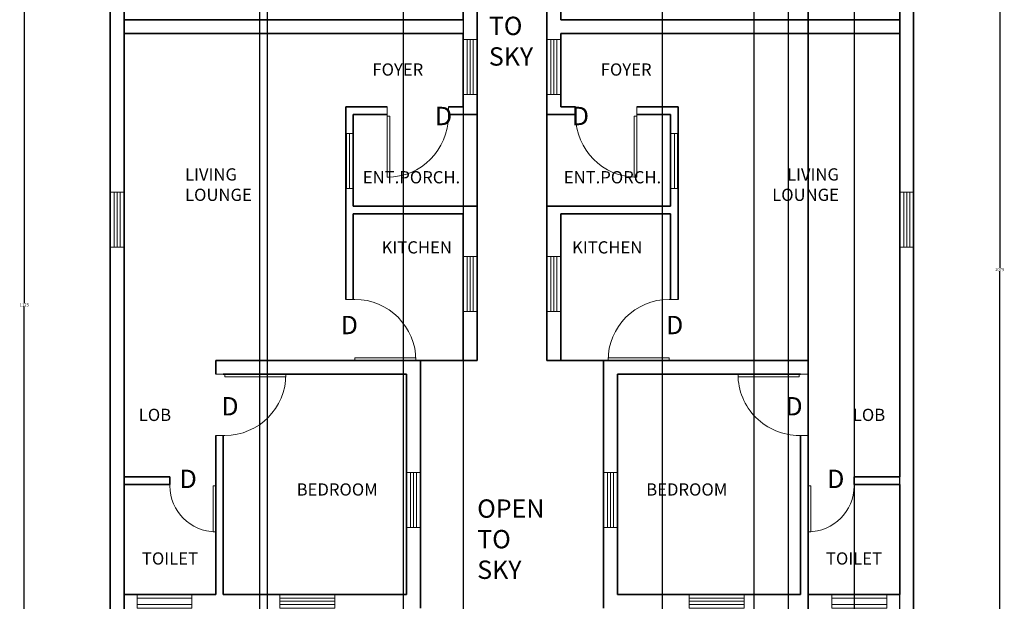
# Model space of a CAD drawing. Units: inches. Extents: x 190 to 836, y -241 to 999.
# Tile 5 of 9: x 191 to 836, y 185 to 566. Entities that reach past the tile are written whole.
import ezdxf

# ---------------------------------------------------------------- set-up
doc = ezdxf.new("R2010")
doc.units = ezdxf.units.IN
doc.header["$MEASUREMENT"] = 0
for name, color, linetype, lineweight in [('A-ANNO-DIMS', 2, 'Continuous', 18), ('A-ANNO-TEXT', 7, 'Continuous', 18), ('A-AREA-IDEN', 7, 'Continuous', 18), ('A-DOOR', 3, 'Continuous', 18), ('A-GLAZ', 4, 'Continuous', 18), ('A-WALL', 7, 'Continuous', 35)]:
    doc.layers.add(name, color=color, linetype=linetype, lineweight=lineweight)
doc.styles.get("Standard").update_dxf_attribs({"font": 'arial.ttf'})
doc.dimstyles.get("Standard").update_dxf_attribs({"dimtxt": 2, "dimasz": 2, "dimexe": 0.18, "dimexo": 0.0625, "dimgap": 0.09, "dimtad": 0, "dimtih": 1, "dimtoh": 1, "dimdec": 0, "dimzin": 0, "dimdsep": 46, "dimlunit": 3, "dimtxsty": 'Standard', "dimcen": 0.09, "dimadec": 0, "dimazin": 0, "dimtfac": 1, "dimtdec": 0, "dimtofl": 0, "dimtmove": 0, "dimatfit": 3, "dimfxl": 1, "dimtolj": 1, "dimtzin": 0, "dimarcsym": 0})

# ---------------------------------------------------------------- blocks, each defined once
blk = doc.blocks.new('*U2')
for p, q in [((0, 0), (0, 6)), ((40, 0), (40, 6))]:
    blk.add_line(p, q)
blk.add_lwpolyline([(0, 0), (0, -40), (1.75, -40), (1.75, 0)], close=True)
blk.add_arc((0, 0), 40, 270, 360)
blk = doc.blocks.new('*U4')
for p, q in [((-40, 0), (-40, 6)), ((0, 0), (0, 6))]:
    blk.add_line(p, q)
blk.add_lwpolyline([(0, 0), (0, -40), (-1.75, -40), (-1.75, 0)], close=True)
blk.add_arc((0, 0), 40, 180, 270)
blk = doc.blocks.new('*U5')
for p, q in [((0, 0), (0, -6)), ((40, 0), (40, -6))]:
    blk.add_line(p, q)
blk.add_lwpolyline([(0, 0), (0, 40), (1.75, 40), (1.75, 0)], close=True)
blk.add_arc((0, 0), 40, 0, 90)
blk = doc.blocks.new('*U3')
for p, q in [((-30, 0), (-30, -6)), ((0, 0), (0, -6))]:
    blk.add_line(p, q)
blk.add_lwpolyline([(0, 0), (0, 30), (-1.75, 30), (-1.75, 0)], close=True)
blk.add_arc((0, 0), 30, 90, 180)
blk = doc.blocks.new('WIN-36IN-9IN-3LINE')
for p, q in [((2.5, 36), (2.5, 0)), ((4.5, 36), (4.5, 0)), ((6.5, 36), (6.5, 0))]:
    blk.add_line(p, q)
blk.add_lwpolyline([(0, 0), (9, 0), (9, 36), (0, 36)], close=True)
blk = doc.blocks.new('WIN-36IN-9IN-2LINE')
for p, q in [((0, 6.5), (36, 6.5)), ((0, 2.5), (36, 2.5))]:
    blk.add_line(p, q)
blk.add_lwpolyline([(36, 0), (36, 9), (0, 9), (0, 0)], close=True)
blk = doc.blocks.new('WIN-36IN-5IN-PARTITION')
for p, q in [((5, 36), (0, 36)), ((0.5, 36), (0.5, 0)), ((2.5, 36), (2.5, 0)), ((5, 0), (5, 36)), ((0, 0), (5, 0))]:
    blk.add_line(p, q)
blk = doc.blocks.new('*D17')
at = {"layer": 'A-ANNO-DIMS', "color": 0, "lineweight": -2, "transparency": 16777216}
for p, q in [((250.38, 941.53), (193.96, 941.53)), ((194.14, 939.53), (194.14, 380.14)), ((194.14, -181.47), (194.14, 377.92)), ((447.38, -183.47), (193.96, -183.47))]:
    blk.add_line(p, q, dxfattribs=at)
at = {"layer": 'A-ANNO-DIMS', "color": 0, "transparency": 16777216}
for points in [[(193.8, 939.53), (194.47, 939.53), (194.14, 941.53)], [(193.8, -181.47), (194.47, -181.47), (194.14, -183.47)]]:
    blk.add_solid(points, dxfattribs=at)
at = {"layer": 'Defpoints', "color": 0, "transparency": 16777216}
for p in [(194.14, 941.53), (250.44, 941.53), (447.44, -183.47)]:
    blk.add_point(p, dxfattribs=at)
at = {"layer": 'A-ANNO-DIMS', "color": 0, "transparency": 16777216, "insert": (194.14, 379.03), "char_height": 2, "attachment_point": 5}
blk.add_mtext('\\A1;1125', dxfattribs=at)
blk = doc.blocks.new('*D18')
at = {"layer": 'A-ANNO-DIMS', "color": 0, "lineweight": -2, "transparency": 16777216}
for p, q in [((776.5, 941.53), (832.94, 941.53)), ((832.76, 939.53), (832.76, 403.14)), ((832.76, -135.47), (832.76, 400.92)), ((776.5, -137.47), (832.94, -137.47))]:
    blk.add_line(p, q, dxfattribs=at)
at = {"layer": 'A-ANNO-DIMS', "color": 0, "transparency": 16777216}
for points in [[(832.43, 939.53), (833.1, 939.53), (832.76, 941.53)], [(832.43, -135.47), (833.1, -135.47), (832.76, -137.47)]]:
    blk.add_solid(points, dxfattribs=at)
at = {"layer": 'Defpoints', "color": 0, "transparency": 16777216}
for p in [(776.44, 941.53), (832.76, 941.53), (776.44, -137.47)]:
    blk.add_point(p, dxfattribs=at)
at = {"layer": 'A-ANNO-DIMS', "color": 0, "transparency": 16777216, "insert": (832.76, 402.03), "char_height": 2, "attachment_point": 5}
blk.add_mtext('\\A1;1079', dxfattribs=at)
blk = doc.blocks.new('*D29')
at = {"layer": 'A-ANNO-DIMS', "color": 0, "lineweight": -2, "transparency": 16777216}
for p, q in [((259.44, 565.47), (259.44, -239.95)), ((481.55, 565.47), (481.55, -239.95)), ((261.44, -239.77), (367.21, -239.77)), ((479.55, -239.77), (373.79, -239.77))]:
    blk.add_line(p, q, dxfattribs=at)
at = {"layer": 'A-ANNO-DIMS', "color": 0, "transparency": 16777216}
for points in [[(261.44, -239.44), (261.44, -240.11), (259.44, -239.77)], [(479.55, -239.44), (479.55, -240.11), (481.55, -239.77)]]:
    blk.add_solid(points, dxfattribs=at)
at = {"layer": 'Defpoints', "color": 0, "transparency": 16777216}
for p in [(259.44, 565.53), (481.55, 565.53), (481.55, -239.77)]:
    blk.add_point(p, dxfattribs=at)
at = {"layer": 'A-ANNO-DIMS', "color": 0, "transparency": 16777216, "insert": (370.5, -239.77), "char_height": 2, "attachment_point": 5}
blk.add_mtext('\\A1;222.1', dxfattribs=at)
blk = doc.blocks.new('*D31')
at = {"layer": 'A-ANNO-DIMS', "color": 0, "lineweight": -2, "transparency": 16777216}
for p, q in [((707.44, 855.47), (707.44, -239.95)), ((737.44, 855.47), (737.44, -239.95)), ((709.44, -239.77), (720.92, -239.77)), ((735.44, -239.77), (723.96, -239.77))]:
    blk.add_line(p, q, dxfattribs=at)
at = {"layer": 'A-ANNO-DIMS', "color": 0, "transparency": 16777216}
for points in [[(709.44, -239.44), (709.44, -240.11), (707.44, -239.77)], [(735.44, -239.44), (735.44, -240.11), (737.44, -239.77)]]:
    blk.add_solid(points, dxfattribs=at)
at = {"layer": 'Defpoints', "color": 0, "transparency": 16777216}
for p in [(707.44, 855.53), (737.44, 855.53), (707.44, -239.77)]:
    blk.add_point(p, dxfattribs=at)
at = {"layer": 'A-ANNO-DIMS', "color": 0, "transparency": 16777216, "insert": (722.44, -239.77), "char_height": 2, "attachment_point": 5}
blk.add_mtext('\\A1;30', dxfattribs=at)
blk = doc.blocks.new('*D35')
at = {"layer": 'A-ANNO-DIMS', "color": 0, "lineweight": -2, "transparency": 16777216}
for p, q in [((259.44, -8.41), (259.44, 998.02)), ((261.44, 997.84), (302.42, 997.84)), ((346.44, 997.84), (305.47, 997.84)), ((348.44, -8.41), (348.44, 998.02))]:
    blk.add_line(p, q, dxfattribs=at)
at = {"layer": 'A-ANNO-DIMS', "color": 0, "transparency": 16777216}
for points in [[(261.44, 998.17), (261.44, 997.5), (259.44, 997.84)], [(346.44, 998.17), (346.44, 997.5), (348.44, 997.84)]]:
    blk.add_solid(points, dxfattribs=at)
at = {"layer": 'Defpoints', "color": 0, "transparency": 16777216}
for p in [(348.44, 997.84), (259.44, -8.47), (348.44, -8.47)]:
    blk.add_point(p, dxfattribs=at)
at = {"layer": 'A-ANNO-DIMS', "color": 0, "transparency": 16777216, "insert": (303.94, 997.84), "char_height": 2, "attachment_point": 5}
blk.add_mtext('\\A1;89', dxfattribs=at)
blk = doc.blocks.new('*D36')
at = {"layer": 'A-ANNO-DIMS', "color": 0, "lineweight": -2, "transparency": 16777216}
for p, q in [((353.44, -8.41), (353.44, 998.02)), ((355.44, 997.84), (396.42, 997.84)), ((440.44, 997.84), (399.47, 997.84)), ((442.44, -8.41), (442.44, 998.02))]:
    blk.add_line(p, q, dxfattribs=at)
at = {"layer": 'A-ANNO-DIMS', "color": 0, "transparency": 16777216}
for points in [[(355.44, 998.17), (355.44, 997.5), (353.44, 997.84)], [(440.44, 998.17), (440.44, 997.5), (442.44, 997.84)]]:
    blk.add_solid(points, dxfattribs=at)
at = {"layer": 'Defpoints', "color": 0, "transparency": 16777216}
for p in [(442.44, 997.84), (353.44, -8.47), (442.44, -8.47)]:
    blk.add_point(p, dxfattribs=at)
at = {"layer": 'A-ANNO-DIMS', "color": 0, "transparency": 16777216, "insert": (397.94, 997.84), "char_height": 2, "attachment_point": 5}
blk.add_mtext('\\A1;89', dxfattribs=at)
blk = doc.blocks.new('*D43')
at = {"layer": 'A-ANNO-DIMS', "color": 0, "lineweight": -2, "transparency": 16777216}
for p, q in [((694.44, -128.41), (694.44, 998.02)), ((696.44, 997.84), (729.43, 997.84)), ((765.44, 997.84), (732.45, 997.84)), ((767.44, -128.41), (767.44, 998.02))]:
    blk.add_line(p, q, dxfattribs=at)
at = {"layer": 'A-ANNO-DIMS', "color": 0, "transparency": 16777216}
for points in [[(696.44, 998.17), (696.44, 997.5), (694.44, 997.84)], [(765.44, 998.17), (765.44, 997.5), (767.44, 997.84)]]:
    blk.add_solid(points, dxfattribs=at)
at = {"layer": 'Defpoints', "color": 0, "transparency": 16777216}
for p in [(767.44, 997.84), (694.44, -128.47), (767.44, -128.47)]:
    blk.add_point(p, dxfattribs=at)
at = {"layer": 'A-ANNO-DIMS', "color": 0, "transparency": 16777216, "insert": (730.94, 997.84), "char_height": 2, "attachment_point": 5}
blk.add_mtext('\\A1;73', dxfattribs=at)
blk = doc.blocks.new('*D45')
at = {"layer": 'A-ANNO-DIMS', "color": 0, "lineweight": -2, "transparency": 16777216}
for p, q in [((612.1, 115.59), (612.1, 998.02)), ((614.1, 997.84), (640.58, 997.84)), ((670.1, 997.84), (643.62, 997.84)), ((672.1, 115.59), (672.1, 998.02))]:
    blk.add_line(p, q, dxfattribs=at)
at = {"layer": 'A-ANNO-DIMS', "color": 0, "transparency": 16777216}
for points in [[(614.1, 998.17), (614.1, 997.5), (612.1, 997.84)], [(670.1, 998.17), (670.1, 997.5), (672.1, 997.84)]]:
    blk.add_solid(points, dxfattribs=at)
at = {"layer": 'Defpoints', "color": 0, "transparency": 16777216}
for p in [(672.1, 997.84), (612.1, 115.53), (672.1, 115.53)]:
    blk.add_point(p, dxfattribs=at)
at = {"layer": 'A-ANNO-DIMS', "color": 0, "transparency": 16777216, "insert": (642.1, 997.84), "char_height": 2, "attachment_point": 5}
blk.add_mtext('\\A1;60', dxfattribs=at)
blk = doc.blocks.new('*D46')
at = {"layer": 'A-ANNO-DIMS', "color": 0, "lineweight": -2, "transparency": 16777216}
for p, q in [((707.44, 120.59), (707.44, 998.02)), ((709.44, 997.84), (735.92, 997.84)), ((765.44, 997.84), (738.97, 997.84)), ((767.44, 120.59), (767.44, 998.02))]:
    blk.add_line(p, q, dxfattribs=at)
at = {"layer": 'A-ANNO-DIMS', "color": 0, "transparency": 16777216}
for points in [[(709.44, 998.17), (709.44, 997.5), (707.44, 997.84)], [(765.44, 998.17), (765.44, 997.5), (767.44, 997.84)]]:
    blk.add_solid(points, dxfattribs=at)
at = {"layer": 'Defpoints', "color": 0, "transparency": 16777216}
for p in [(767.44, 997.84), (707.44, 120.53), (767.44, 120.53)]:
    blk.add_point(p, dxfattribs=at)
at = {"layer": 'A-ANNO-DIMS', "color": 0, "transparency": 16777216, "insert": (737.44, 997.84), "char_height": 2, "attachment_point": 5}
blk.add_mtext('\\A1;60', dxfattribs=at)

msp = doc.modelspace()

# ---------------------------------------------------------------- linework, layer by layer
at = {"layer": 'A-WALL'}
for p, q in [((250.4421, 941.5313), (250.4421, 556.5313)), ((776.4421, 941.5313), (776.4421, 556.5313)), ((259.4421, 855.5313), (259.4421, 565.5313)), ((767.4421, 855.5313), (767.4421, 565.5313)), ((490.5536, 556.5313), (490.5536, 779.5313)), ((536.3307, 556.5313), (536.3307, 779.5313)), ((481.5536, 565.5313), (481.5536, 613.5313)), ((545.3307, 565.5313), (545.3307, 613.5313)), ((250.4421, -137.4687), (250.4421, 565.5313)), ((259.4421, 565.5313), (481.5536, 565.5313)), ((490.5536, 565.5313), (490.5536, 342.5313)), ((536.3307, 565.5313), (536.3307, 342.5313)), ((767.4421, 565.5313), (545.3307, 565.5313)), ((767.4421, 266.5313), (767.4421, 565.5313)), ((776.4421, -8.4687), (776.4421, 565.5313)), ((259.4421, 266.5313), (259.4421, 556.5313)), ((259.4421, 556.5313), (481.5536, 556.5313)), ((481.5536, 556.5313), (481.5536, 508.5313)), ((767.4421, 556.5313), (545.3307, 556.5313)), ((545.3307, 556.5313), (545.3307, 508.5313)), ((767.4421, 266.5313), (767.4421, 556.5313)), ((404.5536, 508.5313), (431.7728, 508.5313)), ((404.5536, 508.5313), (404.5536, 382.5313)), ((409.5536, 503.5313), (428.1141, 503.5313)), ((409.5536, 503.5313), (409.5536, 443.5313)), ((428.1141, 503.5313), (431.7728, 503.5313)), ((471.7728, 508.5313), (481.5536, 508.5313)), ((471.7728, 503.5313), (490.5536, 503.5313)), ((555.1115, 503.5313), (536.3307, 503.5313)), ((555.1115, 508.5313), (545.3307, 508.5313)), ((622.3307, 508.5313), (595.1115, 508.5313)), ((598.7702, 503.5313), (595.1115, 503.5313)), ((617.3307, 503.5313), (598.7702, 503.5313)), ((617.3307, 503.5313), (617.3307, 443.5313)), ((622.3307, 508.5313), (622.3307, 382.5313)), ((409.5536, 443.5313), (490.5536, 443.5313)), ((409.5536, 438.5313), (481.5536, 438.5313)), ((409.5536, 438.5313), (409.5536, 382.5313)), ((481.5536, 438.5313), (481.5536, 342.5313)), ((617.3307, 443.5313), (536.3307, 443.5313)), ((617.3307, 438.5313), (545.3307, 438.5313)), ((545.3307, 438.5313), (545.3307, 342.5313)), ((617.3307, 438.5313), (617.3307, 382.5313)), ((319.4421, 342.5313), (490.5536, 342.5313)), ((319.4421, 342.5313), (319.4421, 333.5313)), ((453.4421, 342.5313), (453.4421, 180.5313)), ((707.4421, 342.5313), (536.3307, 342.5313)), ((573.4421, 342.5313), (573.4421, 180.5313)), ((707.4421, 342.5313), (707.4421, 333.5313)), ((324.4421, 333.5313), (444.4421, 333.5313)), ((444.4421, 333.5313), (444.4421, 189.5313)), ((702.4421, 333.5313), (582.4421, 333.5313)), ((582.4421, 333.5313), (582.4421, 189.5313)), ((319.4421, 293.5313), (319.4421, 189.5313)), ((324.4421, 293.5313), (324.4421, 189.5313)), ((702.4421, 293.5313), (702.4421, 189.5313)), ((707.4421, 293.5313), (707.4421, 189.5313)), ((259.4421, 266.5313), (289.4421, 266.5313)), ((289.4421, 261.5313), (289.4421, 266.5313)), ((767.4421, 266.5313), (737.4421, 266.5313)), ((737.4421, 261.5313), (737.4421, 266.5313)), ((259.4421, 261.5313), (289.4421, 261.5313)), ((259.4421, 189.5313), (259.4421, 261.5313)), ((767.4421, 261.5313), (737.4421, 261.5313)), ((767.4421, 189.5313), (767.4421, 261.5313)), ((767.4421, 189.5313), (767.4421, 261.5313)), ((319.4421, 189.5313), (259.4421, 189.5313)), ((444.4421, 189.5313), (324.4421, 189.5313)), ((582.4421, 189.5313), (702.4421, 189.5313)), ((707.4421, 189.5313), (767.4421, 189.5313))]:
    msp.add_line(p, q, dxfattribs=at)

# ---------------------------------------------------------------- block references
at = {"layer": 'A-DOOR', "xscale": -1}
for name, p, rotation in [('*U5', (431.7728, 502.5313), 180), ('*U4', (410.5536, 342.5313), 90), ('*U2', (325.4421, 333.5313), 90), ('*U3', (319.4421, 260.5313), 180)]:
    msp.add_blockref(name, p, dxfattribs=dict(at, rotation=rotation))
at = {"layer": 'A-DOOR'}
for name, p, rotation in [('*U5', (595.1115, 502.5313), 179.9999999999999), ('*U4', (616.3307, 342.5313), 269.9999999999999), ('*U2', (701.4421, 333.5313), 269.9999999999999), ('*U3', (707.4421, 260.5313), 179.9999999999999)]:
    msp.add_blockref(name, p, dxfattribs=dict(at, rotation=rotation))
at = {"layer": 'A-GLAZ', "extrusion": (0, 0, -1), "zscale": -1}
for name, p, rotation in [('WIN-36IN-9IN-3LINE', (-481.5534, 552.6634), 180), ('WIN-36IN-9IN-3LINE', (-250.442, 452.6202), 180), ('WIN-36IN-9IN-3LINE', (-481.5534, 410.5307), 180), ('WIN-36IN-9IN-3LINE', (-444.442, 269.2117), 180), ('WIN-36IN-9IN-2LINE', (-267.917, 189.5317), 180), ('WIN-36IN-9IN-3LINE', (-397.4358, 189.5315), 269.9999999999998)]:
    msp.add_blockref(name, p, dxfattribs=dict(at, rotation=rotation))
at = {"layer": 'A-GLAZ'}
for name, p, rotation in [('WIN-36IN-9IN-3LINE', (545.3309, 552.6634), 180), ('WIN-36IN-5IN-PARTITION', (622.3303, 491.1627), 180), ('WIN-36IN-9IN-3LINE', (776.4423, 452.6202), 180), ('WIN-36IN-9IN-3LINE', (545.3309, 410.5307), 180), ('WIN-36IN-9IN-3LINE', (582.4423, 269.2117), 180), ('WIN-36IN-9IN-3LINE', (629.4485, 189.5315), 269.9999999999995), ('WIN-36IN-9IN-2LINE', (758.9673, 189.5317), 180)]:
    msp.add_blockref(name, p, dxfattribs=dict(at, rotation=rotation))
msp.add_blockref('WIN-36IN-5IN-PARTITION', (404.554, 455.1627), dxfattribs=at)

# ---------------------------------------------------------------- texts
at = {"layer": 'A-ANNO-TEXT', "char_height": 12}
for insert, attachment_point in [((463.0077, 508.5313), 1), ((563.8765, 508.5313), 3), ((401.3187, 371.7822), 1), ((625.5656, 371.7822), 3), ((323.1618, 318.6312), 1), ((703.7225, 318.6312), 3), ((295.807, 259.1163), 7), ((731.0773, 259.1163), 9)]:
    msp.add_mtext_dynamic_manual_height_columns('D', width=8.765037, gutter_width=1, heights=[0], dxfattribs=dict(at, insert=insert, attachment_point=attachment_point))
at = {"layer": 'A-AREA-IDEN'}
for s, width, insert, char_height, attachment_point in [('OPEN TO SKY', 38.023659, (498.3071, 587.4984), 12, 1), ('FOYER', 33.040256, (422.0497, 528.9458), 8, 7), ('FOYER', 33.040256, (604.8346, 528.9458), 8, 9), ('LIVING LOUNGE ', 33.040256, (299.3596, 446.9767), 8, 7), ('ENT.PORCH.', 33.040256, (415.7534, 458.4672), 8, 7), ('ENT.PORCH.', 33.040256, (611.1309, 458.4672), 8, 9), ('LIVING LOUNGE ', 33.040256, (727.5247, 446.9767), 8, 9), ('KITCHEN', 33.040256, (428.1017, 412.5922), 8, 7), ('KITCHEN', 33.040256, (598.7825, 412.5922), 8, 9), ('LOB', 33.040256, (269.0822, 302.9943), 8, 7), ('LOB', 33.040256, (757.8021, 302.9943), 8, 9), ('BEDROOM', 33.040256, (372.4463, 254.1832), 8, 7), ('BEDROOM', 33.040256, (654.438, 254.1832), 8, 9), ('OPEN TO SKY', 38.023659, (490.688, 251.6786), 12, 1), ('TOILET', 33.040256, (271.1436, 209.0395), 8, 7), ('TOILET', 33.040256, (755.7407, 209.0395), 8, 9)]:
    msp.add_mtext_dynamic_manual_height_columns(s, width=width, gutter_width=1, heights=[0], dxfattribs=dict(at, insert=insert, char_height=char_height, attachment_point=attachment_point))

# ---------------------------------------------------------------- dimensions: what is measured, and where the dimension line sits
at = {"layer": 'A-ANNO-DIMS'}
for base, p1, p2, override, picture, middle in [((348.4421, 997.8363), (259.4421, -8.4687), (348.4421, -8.4687), {"dimdec": 0, "dimlfac": 1, "dimrnd": 0, "dimzin": 0, "dimdsep": 46, "dimlunit": 2}, '*D35', (303.9421, 997.8363)), ((442.4421, 997.8363), (353.4421, -8.4687), (442.4421, -8.4687), {"dimdec": 0, "dimlfac": 1, "dimrnd": 0, "dimzin": 0, "dimdsep": 46, "dimlunit": 2}, '*D36', (397.9421, 997.8363)), ((672.0998, 997.8363), (612.0998, 115.5313), (672.0998, 115.5313), {"dimdec": 0, "dimlfac": 1, "dimrnd": 0, "dimzin": 0, "dimdsep": 46, "dimlunit": 2}, '*D45', (642.0998, 997.8363)), ((767.4421, 997.8363), (694.4376, -128.4687), (767.4421, -128.4687), {"dimdec": 0, "dimlfac": 1, "dimrnd": 0, "dimzin": 0, "dimdsep": 46, "dimlunit": 2}, '*D43', (730.9399, 997.8363)), ((767.4421, 997.8363), (707.4421, 120.5313), (767.4421, 120.5313), {"dimdec": 0, "dimlfac": 1, "dimrnd": 0, "dimzin": 0, "dimdsep": 46, "dimlunit": 2}, '*D46', (737.4421, 997.8363)), ((707.4421, -239.7737), (737.4421, 855.5313), (707.4421, 855.5313), {"dimdec": 0, "dimlfac": 1, "dimrnd": 0, "dimzin": 0, "dimdsep": 46, "dimlunit": 2}, '*D31', (722.4421, -239.7737)), ((481.5536, -239.7737), (259.4421, 565.5313), (481.5536, 565.5313), {"dimdec": 1, "dimlfac": 1, "dimrnd": 0, "dimzin": 0, "dimdsep": 46, "dimlunit": 2}, '*D29', (370.4979, -239.7737))]:
    dim = msp.add_linear_dim(base=base, p1=p1, p2=p2, dimstyle='Standard', override=override, dxfattribs=at)
    dim.commit()
    dim.dimension.update_dxf_attribs({"geometry": picture, "text_midpoint": middle})
for base, p1, p2, picture, middle in [((194.1371, 941.5313), (447.4421, -183.4687), (250.4421, 941.5313), '*D17', (194.1371, 379.0313)), ((832.7634, 941.5313), (776.4421, -137.4687), (776.4421, 941.5313), '*D18', (832.7634, 402.0313))]:
    dim = msp.add_linear_dim(base=base, p1=p1, p2=p2, angle=90, dimstyle='Standard', override={"dimdec": 0, "dimlfac": 1, "dimrnd": 0, "dimzin": 0, "dimdsep": 46, "dimlunit": 2}, dxfattribs=at)
    dim.commit()
    dim.dimension.update_dxf_attribs({"geometry": picture, "text_midpoint": middle})

doc.saveas('drawing.dxf')
